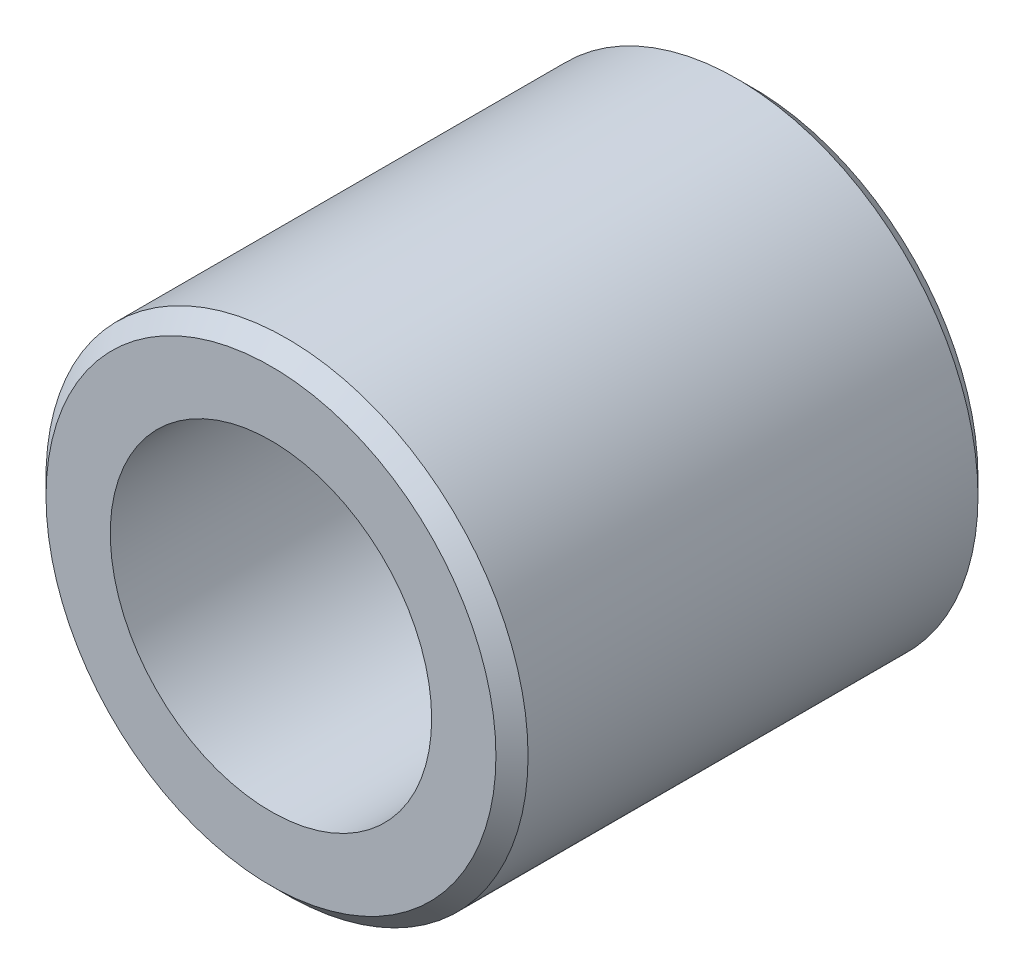
ISO-10303-21;
HEADER;
FILE_DESCRIPTION(('STEP AP214'),'2;1');
FILE_NAME('part.step','',(''),(''),'','','');
FILE_SCHEMA(('AUTOMOTIVE_DESIGN { 1 0 10303 214 1 1 1 1 }'));
ENDSEC;
DATA;
#1=APPLICATION_CONTEXT('core data for automotive mechanical design processes');
#2=APPLICATION_PROTOCOL_DEFINITION('international standard','automotive_design',2000,#1);
#3=PRODUCT_CONTEXT('',#1,'mechanical');
#4=PRODUCT('Part','Part','',(#3));
#5=PRODUCT_RELATED_PRODUCT_CATEGORY('part','',(#4));
#6=PRODUCT_DEFINITION_FORMATION('','',#4);
#7=PRODUCT_DEFINITION_CONTEXT('part definition',#1,'design');
#8=PRODUCT_DEFINITION('design','',#6,#7);
#9=PRODUCT_DEFINITION_SHAPE('','',#8);
#10=(LENGTH_UNIT() NAMED_UNIT(*) SI_UNIT(.MILLI.,.METRE.));
#11=(NAMED_UNIT(*) PLANE_ANGLE_UNIT() SI_UNIT($,.RADIAN.));
#12=(NAMED_UNIT(*) SI_UNIT($,.STERADIAN.) SOLID_ANGLE_UNIT());
#13=UNCERTAINTY_MEASURE_WITH_UNIT(LENGTH_MEASURE(1.E-05),#10,'distance_accuracy_value','');
#14=(GEOMETRIC_REPRESENTATION_CONTEXT(3) GLOBAL_UNCERTAINTY_ASSIGNED_CONTEXT((#13)) GLOBAL_UNIT_ASSIGNED_CONTEXT((#10,
#11,#12)) REPRESENTATION_CONTEXT('',''));
#15=CARTESIAN_POINT('',(0.,0.,0.));
#16=DIRECTION('',(0.,0.,1.));
#17=DIRECTION('',(1.,0.,0.));
#18=AXIS2_PLACEMENT_3D('',#15,#16,#17);
#19=CARTESIAN_POINT('',(0.,0.,15.));
#20=DIRECTION('',(0.,0.,1.));
#21=DIRECTION('',(1.,0.,0.));
#22=AXIS2_PLACEMENT_3D('',#19,#20,#21);
#23=PLANE('',#22);
#24=CARTESIAN_POINT('',(0.,0.,15.));
#25=DIRECTION('',(0.,0.,1.));
#26=DIRECTION('',(1.,0.,0.));
#27=AXIS2_PLACEMENT_3D('',#24,#25,#26);
#28=CIRCLE('',#27,14.);
#29=CARTESIAN_POINT('',(14.,0.,15.));
#30=VERTEX_POINT('',#29);
#31=EDGE_CURVE('E10',#30,#30,#28,.T.);
#32=ORIENTED_EDGE('',*,*,#31,.T.);
#33=EDGE_LOOP('',(#32));
#34=FACE_BOUND('',#33,.T.);
#35=CARTESIAN_POINT('',(0.,0.,15.));
#36=DIRECTION('',(0.,0.,1.));
#37=DIRECTION('',(1.,0.,0.));
#38=AXIS2_PLACEMENT_3D('',#35,#36,#37);
#39=CIRCLE('',#38,10.);
#40=CARTESIAN_POINT('',(10.,0.,15.));
#41=VERTEX_POINT('',#40);
#42=EDGE_CURVE('E66',#41,#41,#39,.T.);
#43=ORIENTED_EDGE('',*,*,#42,.F.);
#44=EDGE_LOOP('',(#43));
#45=FACE_BOUND('',#44,.T.);
#46=ADVANCED_FACE('F44',(#34,#45),#23,.T.);
#47=CARTESIAN_POINT('',(0.,0.,-15.));
#48=DIRECTION('',(0.,0.,1.));
#49=DIRECTION('',(1.,0.,0.));
#50=AXIS2_PLACEMENT_3D('',#47,#48,#49);
#51=PLANE('',#50);
#52=CARTESIAN_POINT('',(0.,0.,-15.));
#53=DIRECTION('',(0.,0.,1.));
#54=DIRECTION('',(1.,0.,0.));
#55=AXIS2_PLACEMENT_3D('',#52,#53,#54);
#56=CIRCLE('',#55,14.);
#57=CARTESIAN_POINT('',(14.,0.,-15.));
#58=VERTEX_POINT('',#57);
#59=EDGE_CURVE('E52',#58,#58,#56,.F.);
#60=ORIENTED_EDGE('',*,*,#59,.T.);
#61=EDGE_LOOP('',(#60));
#62=FACE_BOUND('',#61,.T.);
#63=CARTESIAN_POINT('',(0.,0.,-15.));
#64=DIRECTION('',(0.,0.,1.));
#65=DIRECTION('',(1.,0.,0.));
#66=AXIS2_PLACEMENT_3D('',#63,#64,#65);
#67=CIRCLE('',#66,10.);
#68=CARTESIAN_POINT('',(10.,0.,-15.));
#69=VERTEX_POINT('',#68);
#70=EDGE_CURVE('E70',#69,#69,#67,.T.);
#71=ORIENTED_EDGE('',*,*,#70,.T.);
#72=EDGE_LOOP('',(#71));
#73=FACE_BOUND('',#72,.T.);
#74=ADVANCED_FACE('F80',(#62,#73),#51,.F.);
#75=CARTESIAN_POINT('',(0.,0.,15.));
#76=DIRECTION('',(0.,0.,-1.));
#77=DIRECTION('',(-1.,0.,0.));
#78=AXIS2_PLACEMENT_3D('',#75,#76,#77);
#79=CYLINDRICAL_SURFACE('',#78,15.);
#80=CARTESIAN_POINT('',(0.,0.,-14.));
#81=DIRECTION('',(0.,0.,1.));
#82=DIRECTION('',(1.,0.,0.));
#83=AXIS2_PLACEMENT_3D('',#80,#81,#82);
#84=CIRCLE('',#83,15.);
#85=CARTESIAN_POINT('',(15.,0.,-14.));
#86=VERTEX_POINT('',#85);
#87=EDGE_CURVE('E60',#86,#86,#84,.T.);
#88=ORIENTED_EDGE('',*,*,#87,.T.);
#89=EDGE_LOOP('',(#88));
#90=FACE_BOUND('',#89,.T.);
#91=CARTESIAN_POINT('',(0.,0.,14.));
#92=DIRECTION('',(0.,0.,1.));
#93=DIRECTION('',(1.,0.,0.));
#94=AXIS2_PLACEMENT_3D('',#91,#92,#93);
#95=CIRCLE('',#94,15.);
#96=CARTESIAN_POINT('',(15.,0.,14.));
#97=VERTEX_POINT('',#96);
#98=EDGE_CURVE('E62',#97,#97,#95,.F.);
#99=ORIENTED_EDGE('',*,*,#98,.T.);
#100=EDGE_LOOP('',(#99));
#101=FACE_BOUND('',#100,.T.);
#102=ADVANCED_FACE('F84',(#90,#101),#79,.T.);
#103=CARTESIAN_POINT('',(0.,0.,15.));
#104=DIRECTION('',(0.,0.,-1.));
#105=DIRECTION('',(-1.,0.,0.));
#106=AXIS2_PLACEMENT_3D('',#103,#104,#105);
#107=CYLINDRICAL_SURFACE('',#106,10.);
#108=ORIENTED_EDGE('',*,*,#42,.T.);
#109=EDGE_LOOP('',(#108));
#110=FACE_BOUND('',#109,.T.);
#111=ORIENTED_EDGE('',*,*,#70,.F.);
#112=EDGE_LOOP('',(#111));
#113=FACE_BOUND('',#112,.T.);
#114=ADVANCED_FACE('F74',(#110,#113),#107,.F.);
#115=CARTESIAN_POINT('',(0.,0.,-14.));
#116=DIRECTION('',(0.,0.,1.));
#117=DIRECTION('',(1.,0.,0.));
#118=AXIS2_PLACEMENT_3D('',#115,#116,#117);
#119=CONICAL_SURFACE('',#118,15.,0.785398163397449);
#120=ORIENTED_EDGE('',*,*,#59,.F.);
#121=EDGE_LOOP('',(#120));
#122=FACE_BOUND('',#121,.T.);
#123=ORIENTED_EDGE('',*,*,#87,.F.);
#124=EDGE_LOOP('',(#123));
#125=FACE_BOUND('',#124,.T.);
#126=ADVANCED_FACE('F89',(#122,#125),#119,.T.);
#127=CARTESIAN_POINT('',(0.,0.,15.));
#128=DIRECTION('',(0.,0.,-1.));
#129=DIRECTION('',(-1.,0.,0.));
#130=AXIS2_PLACEMENT_3D('',#127,#128,#129);
#131=CONICAL_SURFACE('',#130,14.,0.785398163397447);
#132=ORIENTED_EDGE('',*,*,#98,.F.);
#133=EDGE_LOOP('',(#132));
#134=FACE_BOUND('',#133,.T.);
#135=ORIENTED_EDGE('',*,*,#31,.F.);
#136=EDGE_LOOP('',(#135));
#137=FACE_BOUND('',#136,.T.);
#138=ADVANCED_FACE('F48',(#134,#137),#131,.T.);
#139=CLOSED_SHELL('',(#46,#74,#102,#114,#126,#138));
#140=MANIFOLD_SOLID_BREP('B2',#139);
#141=ADVANCED_BREP_SHAPE_REPRESENTATION('',(#18,#140),#14);
#142=SHAPE_DEFINITION_REPRESENTATION(#9,#141);
ENDSEC;
END-ISO-10303-21;
